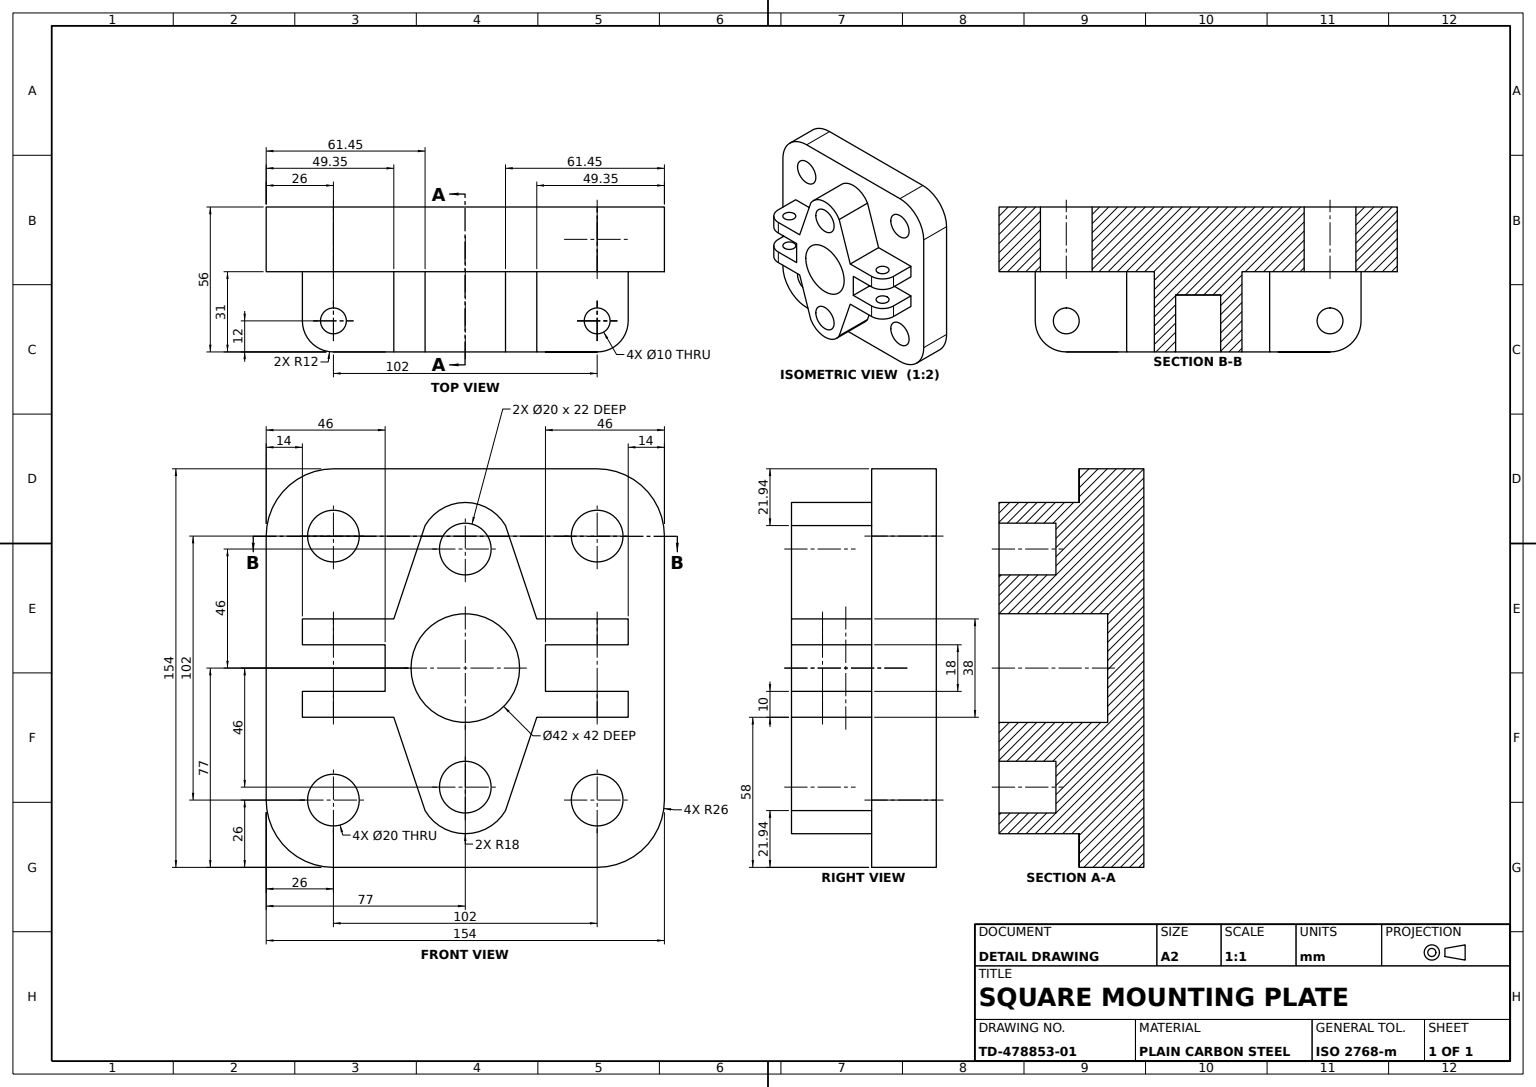
SolidWorks part; units mm, degrees
material "Plain Carbon Steel"
ref_plane "Front Plane" through (0, 0, 0) normal (0, 0, 1) x (1, 0, 0)
ref_plane "Top Plane" through (0, 0, 0) normal (0, 1, 0) x (1, 0, 0)
ref_plane "Right Plane" through (0, 0, 0) normal (1, 0, 0) x (0, 0, -1)
sketch "Base Plate Sketch" plane through (0, 0, 0) normal (0, 0, 1) x (1, 0, 0)
  line L0 (0, -26) -> (0, -128)
  line L1 (26, -154) -> (128, -154)
  line L2 (154, -128) -> (154, -26)
  line L3 (128, 0) -> (26, 0)
  arc A0 (0, -128) -> (26, -154) centre (26, -128) ccw
  arc A1 (128, -154) -> (154, -128) centre (128, -128) ccw
  arc A2 (128, 0) -> (154, -26) centre (128, -26) cw
  arc A3 (26, 0) -> (0, -26) centre (26, -26) ccw
  point P13 (0, 0)
  dimension "D1" = 26
  dimension "D2" = 154
  dimension "D3" = 102
extrude "Base Plate" add sketch "Base Plate Sketch" along normal blind 25
sketch "Flange Boss Sketch" plane through (0, 0, 25) normal (0, 0, 1) x (1, 0, 0)
  line L0 (49.3536, -96) -> (61.4473, -132.0616)
  line L1 (14, -58) -> (49.3536, -58)
  line L2 (46, -68) -> (14, -68)
  line L4 (46, -77) -> (46, -68)
  line L5 (46, -68) -> (46, -86)
  line L7 (108, -86) -> (108, -68)
  line L9 (14, -68) -> (14, -58)
  line L10 (49.3536, -58) -> (61.4473, -21.9384)
  line L11 (104.6464, -58) -> (92.5527, -21.9384)
  line L12 (104.6464, -96) -> (92.5527, -132.0616)
  line L13 (46, -86) -> (14, -86)
  line L14 (14, -86) -> (14, -96)
  line L15 (14, -96) -> (49.3536, -96)
  line L16 (108, -68) -> (140, -68)
  line L17 (140, -68) -> (140, -58)
  line L18 (140, -58) -> (104.6464, -58)
  line L19 (108, -86) -> (140, -86)
  line L20 (140, -86) -> (140, -96)
  line L21 (140, -96) -> (104.6464, -96)
  line L22 (154, -128) -> (154, -26) construction
  line L23 (26, -154) -> (128, -154) construction
  arc A1 (61.4473, -132.0616) -> (92.5527, -132.0616) centre (77, -123) ccw
  arc A2 (92.5527, -21.9384) -> (61.4473, -21.9384) centre (77, -31) ccw
  dimension "D1" = 18
  dimension "D2" = 14
  dimension "D3" = 46
  dimension "D4" = 49.3536
  dimension "D5" = 61.4473
  dimension "D6" = 77
  dimension "D7" = 21.9384
  dimension "D8" = 58
  dimension "D9" = 77
extrude "Flange Boss" add sketch "Flange Boss Sketch" along normal blind 31 contours L11 A2 L10 L1 L9 L2 L4 L5 L13 L14 L15 L0 A1 L12 L21 L20 L19 L7 L16 L17 L18
sketch "Lug Slot 1 Sketch" plane through (0, -96, 0) normal (0, -1, 0) x (1, 0, 0)
  line L0 (140, 56) -> (140, 44)
  line L1 (140, 56) -> (140, 25) construction
  line L3 (140, 56) -> (128, 56)
  arc A0 (140, 44) -> (128, 56) centre (128, 44) ccw
  dimension "D1" = 12
extrude "Lug Slot 1" cut sketch "Lug Slot 1 Sketch" against normal blind 50
sketch "Lug Slot 2 Sketch" plane through (0, -96, 0) normal (0, -1, 0) x (1, 0, 0)
  line L0 (14, 56) -> (26, 56)
  line L1 (14, 56) -> (49.3536, 56) construction
  line L3 (14, 56) -> (14, 44)
  arc A0 (26, 56) -> (14, 44) centre (26, 44) ccw
  dimension "D1" = 12
extrude "Lug Slot 2" cut sketch "Lug Slot 2 Sketch" against normal blind 50
sketch "Lug Pin Holes Sketch" plane through (0, -96, 0) normal (0, -1, 0) x (1, 0, 0)
  circle A0 centre (128, 44) radius 5
  circle A1 centre (26, 44) radius 5
  dimension "D1" = 10
extrude "Lug Pin Holes 2x" cut sketch "Lug Pin Holes Sketch" against normal blind 50
sketch "Flange Holes Sketch" plane through (0, 0, 56) normal (0, 0, 1) x (1, 0, 0)
  circle A0 centre (77, -31) radius 10
  circle A1 centre (77, -123) radius 10
  dimension "D1" = 20
extrude "Flange Holes 2x" cut sketch "Flange Holes Sketch" against normal blind 22
sketch "Centre Bore Sketch" plane through (0, 0, 56) normal (0, 0, 1) x (1, 0, 0)
  line L0 (26, -86) -> (26, -96) construction
  line L1 (26, -96) -> (49.3536, -96) construction
  circle A1 centre (77, -77) radius 21
  dimension "D1" = 42
  dimension "D2" = 42
  dimension "D3" = 51
  dimension "D4" = 19
extrude "Centre Bore Ø42" cut sketch "Centre Bore Sketch" against normal blind 42
sketch "Corner Holes Sketch" plane through (0, 0, 25) normal (0, 0, 1) x (1, 0, 0)
  circle A0 centre (26, -26) radius 10
  circle A1 centre (128, -26) radius 10
  circle A2 centre (128, -128) radius 10
  circle A3 centre (26, -128) radius 10
  dimension "D1" = 20
  dimension "D2" = 20
  dimension "D3" = 20
  dimension "D4" = 20
  dimension "D5" = 20
extrude "Corner Holes 4xØ20" cut sketch "Corner Holes Sketch" against normal blind 42
